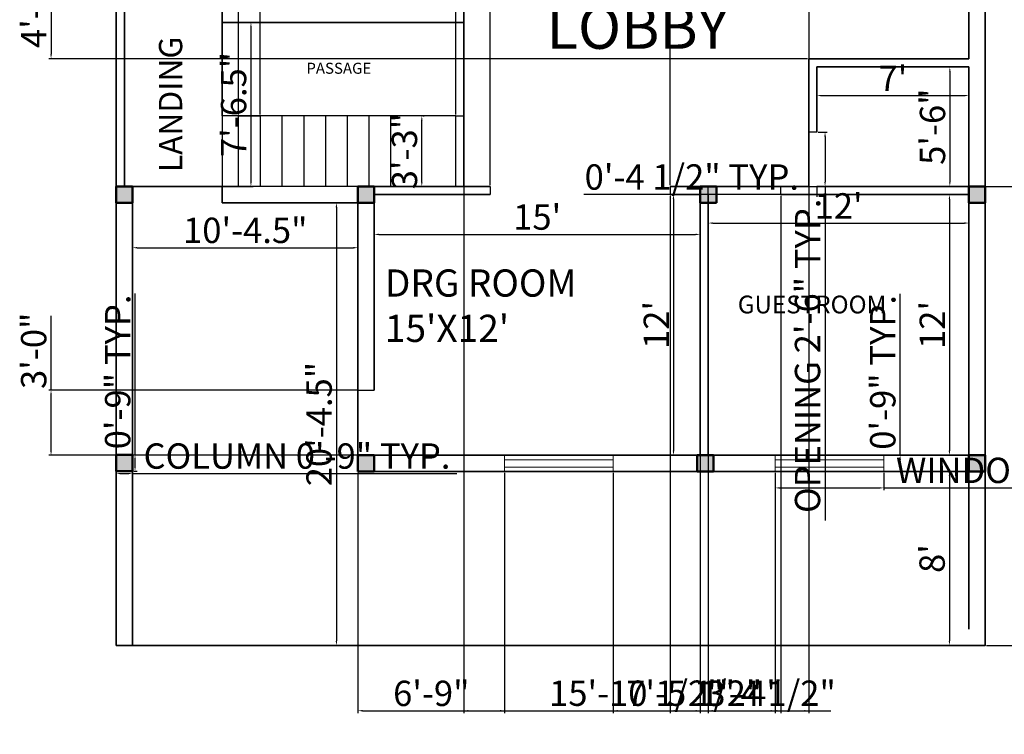
# Model space of a CAD drawing. Units: inches. Extents: x 3316 to 4157, y 2203 to 2977.
# Tile 1 of 4: x 3316 to 3860, y 2203 to 2597. Entities that reach past the tile are written whole.
import ezdxf

# ---------------------------------------------------------------- set-up
doc = ezdxf.new("R2010")
doc.units = ezdxf.units.IN
for name, color, linetype, lineweight in [('A-ANNO-DIMS', 2, 'Continuous', 18), ('A-AREA-IDEN', 7, 'Continuous', 25), ('A-COLS', 7, 'Continuous', 50), ('A-COLS-PATT', 4, 'Continuous', 13), ('A-DOOR', 3, 'Continuous', 25), ('A-FLOR-STRS', 7, 'Continuous', 25), ('A-GLAZ', 4, 'Continuous', 18), ('A-WALL', 7, 'Continuous', 35), ('C-PROP', 7, 'Continuous', 35)]:
    doc.layers.add(name, color=color, linetype=linetype, lineweight=lineweight)
doc.styles.get("Standard").update_dxf_attribs({"font": 'arial.ttf'})
doc.dimstyles.new('ISO-25', dxfattribs={"dimtxt": 14, "dimasz": 2.5, "dimexe": 1.25, "dimexo": 0.625, "dimtad": 1, "dimlunit": 3, "dimtxsty": 'Standard', "dimcen": 2.5, "dimadec": 0, "dimazin": 0, "dimtfac": 1, "dimtmove": 0, "dimatfit": 3, "dimfxl": 1, "dimarcsym": 0})

# ---------------------------------------------------------------- blocks, each defined once
blk = doc.blocks.new('*D4')
at = {"layer": 'A-ANNO-DIMS', "color": 0, "lineweight": -2, "transparency": 16777216}
for p, q in [((3829.8, 2345.34), (3829.8, 2254.34)), ((3830.42, 2347.84), (3831.05, 2347.84)), ((3826.44, 2251.84), (3831.05, 2251.84))]:
    blk.add_line(p, q, dxfattribs=at)
at = {"layer": 'A-ANNO-DIMS', "color": 0, "transparency": 16777216}
for points in [[(3829.38, 2345.34), (3830.21, 2345.34), (3829.8, 2347.84)], [(3829.38, 2254.34), (3830.21, 2254.34), (3829.8, 2251.84)]]:
    blk.add_solid(points, dxfattribs=at)
at = {"layer": 'Defpoints', "color": 0, "transparency": 16777216}
for p in [(3829.8, 2347.84), (3825.82, 2251.84), (3829.8, 2251.84)]:
    blk.add_point(p, dxfattribs=at)
at = {"layer": 'A-ANNO-DIMS', "color": 0, "transparency": 16777216, "insert": (3822.02, 2299.84), "char_height": 14, "attachment_point": 5, "rotation": 90}
blk.add_mtext("8'", dxfattribs=at)
blk = doc.blocks.new('*D5')
at = {"layer": 'A-ANNO-DIMS', "color": 0, "lineweight": -2, "transparency": 16777216}
for p, q in [((3677.36, 2498.34), (3677.36, 2359.34)), ((3677.99, 2500.84), (3678.61, 2500.84)), ((3532.24, 2356.84), (3678.61, 2356.84))]:
    blk.add_line(p, q, dxfattribs=at)
at = {"layer": 'A-ANNO-DIMS', "color": 0, "transparency": 16777216}
for points in [[(3676.94, 2498.34), (3677.78, 2498.34), (3677.36, 2500.84)], [(3676.94, 2359.34), (3677.78, 2359.34), (3677.36, 2356.84)]]:
    blk.add_solid(points, dxfattribs=at)
at = {"layer": 'Defpoints', "color": 0, "transparency": 16777216}
for p in [(3677.36, 2500.84), (3531.62, 2356.84), (3677.36, 2356.84)]:
    blk.add_point(p, dxfattribs=at)
at = {"layer": 'A-ANNO-DIMS', "color": 0, "transparency": 16777216, "insert": (3669.71, 2428.84), "char_height": 14, "attachment_point": 5, "rotation": 90}
blk.add_mtext("12'", dxfattribs=at)
blk = doc.blocks.new('*D7')
at = {"layer": 'A-ANNO-DIMS', "color": 0, "lineweight": -2, "transparency": 16777216}
for p, q in [((3850.21, 2887.84), (4040.36, 2887.84)), ((4039.11, 2885.34), (4039.11, 2254.34)), ((3850.21, 2251.84), (4040.36, 2251.84))]:
    blk.add_line(p, q, dxfattribs=at)
at = {"layer": 'A-ANNO-DIMS', "color": 0, "transparency": 16777216}
for points in [[(4038.69, 2885.34), (4039.53, 2885.34), (4039.11, 2887.84)], [(4038.69, 2254.34), (4039.53, 2254.34), (4039.11, 2251.84)]]:
    blk.add_solid(points, dxfattribs=at)
at = {"layer": 'Defpoints', "color": 0, "transparency": 16777216}
for p in [(3849.58, 2887.84), (3849.58, 2251.84), (4039.11, 2251.84)]:
    blk.add_point(p, dxfattribs=at)
at = {"layer": 'A-ANNO-DIMS', "color": 0, "transparency": 16777216, "insert": (4031.33, 2569.84), "char_height": 14, "attachment_point": 5, "rotation": 90}
blk.add_mtext("53'", dxfattribs=at)
blk = doc.blocks.new('*D12')
at = {"layer": 'A-ANNO-DIMS', "color": 0, "lineweight": -2, "transparency": 16777216}
for p, q in [((3538.33, 2507.84), (3538.33, 2541.84)), ((3538.96, 2544.34), (3539.58, 2544.34)), ((3538.96, 2505.34), (3539.58, 2505.34))]:
    blk.add_line(p, q, dxfattribs=at)
at = {"layer": 'A-ANNO-DIMS', "color": 0, "transparency": 16777216}
for points in [[(3537.91, 2541.84), (3538.75, 2541.84), (3538.33, 2544.34)], [(3537.91, 2507.84), (3538.75, 2507.84), (3538.33, 2505.34)]]:
    blk.add_solid(points, dxfattribs=at)
at = {"layer": 'Defpoints', "color": 0, "transparency": 16777216}
for p in [(3538.33, 2544.34), (3538.33, 2544.34), (3538.33, 2505.34)]:
    blk.add_point(p, dxfattribs=at)
at = {"layer": 'A-ANNO-DIMS', "color": 0, "transparency": 16777216, "insert": (3530.55, 2524.84), "char_height": 14, "attachment_point": 5, "rotation": 90}
blk.add_mtext('3\'-3"', dxfattribs=at)
blk = doc.blocks.new('*D13')
at = {"layer": 'A-ANNO-DIMS', "color": 0, "lineweight": -2, "transparency": 16777216}
for p, q in [((3428.71, 2595.84), (3445.21, 2595.84)), ((3443.96, 2593.34), (3443.96, 2507.84)), ((3428.71, 2505.34), (3445.21, 2505.34))]:
    blk.add_line(p, q, dxfattribs=at)
at = {"layer": 'A-ANNO-DIMS', "color": 0, "transparency": 16777216}
for points in [[(3443.54, 2593.34), (3444.37, 2593.34), (3443.96, 2595.84)], [(3443.54, 2507.84), (3444.37, 2507.84), (3443.96, 2505.34)]]:
    blk.add_solid(points, dxfattribs=at)
at = {"layer": 'Defpoints', "color": 0, "transparency": 16777216}
for p in [(3428.08, 2595.84), (3428.08, 2505.34), (3443.96, 2505.34)]:
    blk.add_point(p, dxfattribs=at)
at = {"layer": 'A-ANNO-DIMS', "color": 0, "transparency": 16777216, "insert": (3436.19, 2550.59), "char_height": 14, "attachment_point": 5, "rotation": 90}
blk.add_mtext('7\'-6.5"', dxfattribs=at)
blk = doc.blocks.new('*D18')
at = {"layer": 'A-ANNO-DIMS', "color": 0, "lineweight": -2, "transparency": 16777216}
for p, q in [((3839.96, 2571.34), (3828.76, 2571.34)), ((3830.01, 2568.84), (3830.01, 2507.84)), ((3839.96, 2505.34), (3828.76, 2505.34))]:
    blk.add_line(p, q, dxfattribs=at)
at = {"layer": 'A-ANNO-DIMS', "color": 0, "transparency": 16777216}
for points in [[(3829.59, 2568.84), (3830.42, 2568.84), (3830.01, 2571.34)], [(3829.59, 2507.84), (3830.42, 2507.84), (3830.01, 2505.34)]]:
    blk.add_solid(points, dxfattribs=at)
at = {"layer": 'Defpoints', "color": 0, "transparency": 16777216}
for p in [(3840.58, 2571.34), (3830.01, 2505.34), (3840.58, 2505.34)]:
    blk.add_point(p, dxfattribs=at)
at = {"layer": 'A-ANNO-DIMS', "color": 0, "transparency": 16777216, "insert": (3822.24, 2538.34), "char_height": 14, "attachment_point": 5, "rotation": 90}
blk.add_mtext('5\'-6"', dxfattribs=at)
blk = doc.blocks.new('*D19')
at = {"layer": 'A-ANNO-DIMS', "color": 0, "lineweight": -2, "transparency": 16777216}
for p, q in [((3756.58, 2570.72), (3756.58, 2554.25)), ((3840.58, 2570.72), (3840.58, 2554.25)), ((3759.08, 2555.5), (3838.08, 2555.5))]:
    blk.add_line(p, q, dxfattribs=at)
at = {"layer": 'A-ANNO-DIMS', "color": 0, "transparency": 16777216}
for points in [[(3759.08, 2555.91), (3759.08, 2555.08), (3756.58, 2555.5)], [(3838.08, 2555.91), (3838.08, 2555.08), (3840.58, 2555.5)]]:
    blk.add_solid(points, dxfattribs=at)
at = {"layer": 'Defpoints', "color": 0, "transparency": 16777216}
for p in [(3756.58, 2571.34), (3840.58, 2571.34), (3840.58, 2555.5)]:
    blk.add_point(p, dxfattribs=at)
at = {"layer": 'A-ANNO-DIMS', "color": 0, "transparency": 16777216, "insert": (3798.58, 2563.12), "char_height": 14, "attachment_point": 5}
blk.add_mtext("7'", dxfattribs=at)
blk = doc.blocks.new('*D20')
at = {"layer": 'A-ANNO-DIMS', "color": 0, "lineweight": -2, "transparency": 16777216}
for p, q in [((3839.96, 2500.84), (3828.55, 2500.84)), ((3829.8, 2498.34), (3829.8, 2359.34)), ((3839.96, 2356.84), (3828.55, 2356.84))]:
    blk.add_line(p, q, dxfattribs=at)
at = {"layer": 'A-ANNO-DIMS', "color": 0, "transparency": 16777216}
for points in [[(3829.38, 2498.34), (3830.21, 2498.34), (3829.8, 2500.84)], [(3829.38, 2359.34), (3830.21, 2359.34), (3829.8, 2356.84)]]:
    blk.add_solid(points, dxfattribs=at)
at = {"layer": 'Defpoints', "color": 0, "transparency": 16777216}
for p in [(3840.58, 2500.84), (3829.8, 2356.84), (3840.58, 2356.84)]:
    blk.add_point(p, dxfattribs=at)
at = {"layer": 'A-ANNO-DIMS', "color": 0, "transparency": 16777216, "insert": (3822.14, 2428.84), "char_height": 14, "attachment_point": 5, "rotation": 90}
blk.add_mtext("12'", dxfattribs=at)
blk = doc.blocks.new('*D21')
at = {"layer": 'A-ANNO-DIMS', "color": 0, "lineweight": -2, "transparency": 16777216}
for p, q in [((3696.58, 2357.47), (3696.58, 2486.34)), ((3840.58, 2357.47), (3840.58, 2486.34)), ((3699.08, 2485.09), (3838.08, 2485.09))]:
    blk.add_line(p, q, dxfattribs=at)
at = {"layer": 'A-ANNO-DIMS', "color": 0, "transparency": 16777216}
for points in [[(3699.08, 2485.51), (3699.08, 2484.68), (3696.58, 2485.09)], [(3838.08, 2485.51), (3838.08, 2484.68), (3840.58, 2485.09)]]:
    blk.add_solid(points, dxfattribs=at)
at = {"layer": 'Defpoints', "color": 0, "transparency": 16777216}
for p in [(3840.58, 2485.09), (3696.58, 2356.84), (3840.58, 2356.84)]:
    blk.add_point(p, dxfattribs=at)
at = {"layer": 'A-ANNO-DIMS', "color": 0, "transparency": 16777216, "insert": (3768.58, 2492.75), "char_height": 14, "attachment_point": 5}
blk.add_mtext("12'", dxfattribs=at)
blk = doc.blocks.new('*D24')
at = {"layer": 'A-ANNO-DIMS', "color": 0, "lineweight": -2, "transparency": 16777216}
for p, q in [((3378.58, 2504.72), (3378.58, 2470.22)), ((3503.08, 2495.72), (3503.08, 2470.22)), ((3381.08, 2471.47), (3500.58, 2471.47))]:
    blk.add_line(p, q, dxfattribs=at)
at = {"layer": 'A-ANNO-DIMS', "color": 0, "transparency": 16777216}
for points in [[(3381.08, 2471.89), (3381.08, 2471.06), (3378.58, 2471.47)], [(3500.58, 2471.89), (3500.58, 2471.06), (3503.08, 2471.47)]]:
    blk.add_solid(points, dxfattribs=at)
at = {"layer": 'Defpoints', "color": 0, "transparency": 16777216}
for p in [(3378.58, 2505.34), (3503.08, 2496.34), (3503.08, 2471.47)]:
    blk.add_point(p, dxfattribs=at)
at = {"layer": 'A-ANNO-DIMS', "color": 0, "transparency": 16777216, "insert": (3440.83, 2479.25), "char_height": 14, "attachment_point": 5}
blk.add_mtext('10\'-4.5"', dxfattribs=at)
blk = doc.blocks.new('*D25')
at = {"layer": 'A-ANNO-DIMS', "color": 0, "lineweight": -2, "transparency": 16777216}
for p, q in [((3502.46, 2496.34), (3489.92, 2496.34)), ((3491.17, 2493.84), (3491.17, 2254.34)), ((3502.46, 2251.84), (3489.92, 2251.84))]:
    blk.add_line(p, q, dxfattribs=at)
at = {"layer": 'A-ANNO-DIMS', "color": 0, "transparency": 16777216}
for points in [[(3490.75, 2493.84), (3491.59, 2493.84), (3491.17, 2496.34)], [(3490.75, 2254.34), (3491.59, 2254.34), (3491.17, 2251.84)]]:
    blk.add_solid(points, dxfattribs=at)
at = {"layer": 'Defpoints', "color": 0, "transparency": 16777216}
for p in [(3503.08, 2496.34), (3491.17, 2251.84), (3503.08, 2251.84)]:
    blk.add_point(p, dxfattribs=at)
at = {"layer": 'A-ANNO-DIMS', "color": 0, "transparency": 16777216, "insert": (3483.4, 2374.09), "char_height": 14, "attachment_point": 5, "rotation": 90}
blk.add_mtext('20\'-4.5"', dxfattribs=at)
blk = doc.blocks.new('*D27')
at = {"layer": 'A-ANNO-DIMS', "color": 0, "lineweight": -2, "transparency": 16777216}
for p, q in [((3512.08, 2500.22), (3512.08, 2477.57)), ((3692.08, 2500.22), (3692.08, 2477.57)), ((3514.58, 2478.82), (3689.58, 2478.82))]:
    blk.add_line(p, q, dxfattribs=at)
at = {"layer": 'A-ANNO-DIMS', "color": 0, "transparency": 16777216}
for points in [[(3514.58, 2479.24), (3514.58, 2478.4), (3512.08, 2478.82)], [(3689.58, 2479.24), (3689.58, 2478.4), (3692.08, 2478.82)]]:
    blk.add_solid(points, dxfattribs=at)
at = {"layer": 'Defpoints', "color": 0, "transparency": 16777216}
for p in [(3512.08, 2500.84), (3692.08, 2500.84), (3692.08, 2478.82)]:
    blk.add_point(p, dxfattribs=at)
at = {"layer": 'A-ANNO-DIMS', "color": 0, "transparency": 16777216, "insert": (3602.08, 2486.59), "char_height": 14, "attachment_point": 5}
blk.add_mtext("15'", dxfattribs=at)
blk = doc.blocks.new('COL-9IN-SQ')
for p, q in [((0, 9), (0, 0)), ((9, 9), (0, 9)), ((9, 0), (9, 9)), ((0, 0), (9, 0))]:
    blk.add_line(p, q)
blk = doc.blocks.new('WIN-60IN')
for p, q in [((0, 0), (0, 9)), ((60, 6.5), (0, 6.5)), ((60, 9), (60, 0)), ((60, 2.5), (0, 2.5)), ((60, 0), (0, 0))]:
    blk.add_line(p, q)
blk = doc.blocks.new('DOOR-30IN-OPENING')
for p, q in [((4.5, 30), (0, 30)), ((4.5, 0), (4.5, 30)), ((0, 0), (4.5, 0))]:
    blk.add_line(p, q)
blk = doc.blocks.new('*D34')
at = {"layer": 'A-ANNO-DIMS', "color": 0, "lineweight": -2, "transparency": 16777216}
for p, q in [((3369.58, 2347.48), (3369.58, 2345.5)), ((3372.08, 2346.75), (3376.08, 2346.75)), ((3378.58, 2347.48), (3378.58, 2345.5)), ((3378.58, 2346.75), (3557.7, 2346.75))]:
    blk.add_line(p, q, dxfattribs=at)
at = {"layer": 'A-ANNO-DIMS', "color": 0, "transparency": 16777216}
for points in [[(3372.08, 2347.17), (3372.08, 2346.34), (3369.58, 2346.75)], [(3376.08, 2347.17), (3376.08, 2346.34), (3378.58, 2346.75)]]:
    blk.add_solid(points, dxfattribs=at)
at = {"layer": 'Defpoints', "color": 0, "transparency": 16777216}
for p in [(3369.58, 2348.1), (3378.58, 2348.1), (3378.58, 2346.75)]:
    blk.add_point(p, dxfattribs=at)
at = {"layer": 'A-ANNO-DIMS', "color": 0, "transparency": 16777216, "insert": (3469.39, 2354.62), "char_height": 14, "attachment_point": 5}
blk.add_mtext('COLUMN 0\'-9" TYP.', dxfattribs=at)
blk = doc.blocks.new('*D35')
at = {"layer": 'A-ANNO-DIMS', "color": 0, "lineweight": -2, "transparency": 16777216}
for p, q in [((3379.93, 2357.1), (3379.93, 2446.19)), ((3379.21, 2357.1), (3381.18, 2357.1)), ((3379.93, 2350.6), (3379.93, 2354.6)), ((3379.21, 2348.1), (3381.18, 2348.1))]:
    blk.add_line(p, q, dxfattribs=at)
at = {"layer": 'A-ANNO-DIMS', "color": 0, "transparency": 16777216}
for points in [[(3379.52, 2354.6), (3380.35, 2354.6), (3379.93, 2357.1)], [(3379.52, 2350.6), (3380.35, 2350.6), (3379.93, 2348.1)]]:
    blk.add_solid(points, dxfattribs=at)
at = {"layer": 'Defpoints', "color": 0, "transparency": 16777216}
for p in [(3378.58, 2357.1), (3379.93, 2357.1), (3378.58, 2348.1)]:
    blk.add_point(p, dxfattribs=at)
at = {"layer": 'A-ANNO-DIMS', "color": 0, "transparency": 16777216, "insert": (3372.16, 2402.9), "char_height": 14, "attachment_point": 5, "rotation": 90}
blk.add_mtext('0\'-9" TYP.', dxfattribs=at)
blk = doc.blocks.new('*D38')
at = {"layer": 'A-ANNO-DIMS', "color": 0, "lineweight": -2, "transparency": 16777216}
for p, q in [((3733.56, 2347.22), (3733.56, 2337.59)), ((3793.56, 2347.22), (3793.56, 2337.59)), ((3736.06, 2338.84), (3791.06, 2338.84)), ((3793.56, 2338.84), (3974.47, 2338.84))]:
    blk.add_line(p, q, dxfattribs=at)
at = {"layer": 'A-ANNO-DIMS', "color": 0, "transparency": 16777216}
for points in [[(3736.06, 2339.26), (3736.06, 2338.43), (3733.56, 2338.84)], [(3791.06, 2339.26), (3791.06, 2338.43), (3793.56, 2338.84)]]:
    blk.add_solid(points, dxfattribs=at)
at = {"layer": 'Defpoints', "color": 0, "transparency": 16777216}
for p in [(3733.56, 2347.84), (3793.56, 2347.84), (3793.56, 2338.84)]:
    blk.add_point(p, dxfattribs=at)
at = {"layer": 'A-ANNO-DIMS', "color": 0, "transparency": 16777216, "insert": (3885.26, 2346.71), "char_height": 14, "attachment_point": 5}
blk.add_mtext('WINDOW 5\'-0" TYP.', dxfattribs=at)
blk = doc.blocks.new('*D39')
at = {"layer": 'A-ANNO-DIMS', "color": 0, "lineweight": -2, "transparency": 16777216}
for p, q in [((3802.56, 2356.84), (3802.56, 2445.93)), ((3794.18, 2356.84), (3803.81, 2356.84)), ((3802.56, 2350.34), (3802.56, 2354.34)), ((3794.18, 2347.84), (3803.81, 2347.84))]:
    blk.add_line(p, q, dxfattribs=at)
at = {"layer": 'A-ANNO-DIMS', "color": 0, "transparency": 16777216}
for points in [[(3802.14, 2354.34), (3802.98, 2354.34), (3802.56, 2356.84)], [(3802.14, 2350.34), (3802.98, 2350.34), (3802.56, 2347.84)]]:
    blk.add_solid(points, dxfattribs=at)
at = {"layer": 'Defpoints', "color": 0, "transparency": 16777216}
for p in [(3793.56, 2356.84), (3802.56, 2356.84), (3793.56, 2347.84)]:
    blk.add_point(p, dxfattribs=at)
at = {"layer": 'A-ANNO-DIMS', "color": 0, "transparency": 16777216, "insert": (3794.79, 2402.64), "char_height": 14, "attachment_point": 5, "rotation": 90}
blk.add_mtext('0\'-9" TYP.', dxfattribs=at)
blk = doc.blocks.new('*D44')
at = {"layer": 'A-ANNO-DIMS', "color": 0, "lineweight": -2, "transparency": 16777216}
for p, q in [((3757.21, 2535.34), (3762.33, 2535.34)), ((3761.08, 2532.84), (3761.08, 2507.84)), ((3757.21, 2505.34), (3762.33, 2505.34)), ((3761.08, 2505.34), (3761.08, 2320.76))]:
    blk.add_line(p, q, dxfattribs=at)
at = {"layer": 'A-ANNO-DIMS', "color": 0, "transparency": 16777216}
for points in [[(3760.67, 2532.84), (3761.5, 2532.84), (3761.08, 2535.34)], [(3760.67, 2507.84), (3761.5, 2507.84), (3761.08, 2505.34)]]:
    blk.add_solid(points, dxfattribs=at)
at = {"layer": 'Defpoints', "color": 0, "transparency": 16777216}
for p in [(3756.58, 2535.34), (3756.58, 2505.34), (3761.08, 2505.34)]:
    blk.add_point(p, dxfattribs=at)
at = {"layer": 'A-ANNO-DIMS', "color": 0, "transparency": 16777216, "insert": (3753.22, 2411.8), "char_height": 14, "attachment_point": 5, "rotation": 90}
blk.add_mtext('OPENING 2\'-6" TYP.', dxfattribs=at)
blk = doc.blocks.new('*D45')
at = {"layer": 'A-ANNO-DIMS', "color": 0, "lineweight": -2, "transparency": 16777216}
for p, q in [((3752.08, 2504.72), (3752.08, 2499.59)), ((3756.58, 2504.72), (3756.58, 2499.59)), ((3749.58, 2500.84), (3627.87, 2500.84)), ((3756.58, 2500.84), (3752.08, 2500.84)), ((3759.08, 2500.84), (3761.58, 2500.84))]:
    blk.add_line(p, q, dxfattribs=at)
at = {"layer": 'A-ANNO-DIMS', "color": 0, "transparency": 16777216}
for points in [[(3749.58, 2501.26), (3749.58, 2500.43), (3752.08, 2500.84)], [(3759.08, 2501.26), (3759.08, 2500.43), (3756.58, 2500.84)]]:
    blk.add_solid(points, dxfattribs=at)
at = {"layer": 'Defpoints', "color": 0, "transparency": 16777216}
for p in [(3752.08, 2505.34), (3756.58, 2505.34), (3752.08, 2500.84)]:
    blk.add_point(p, dxfattribs=at)
at = {"layer": 'A-ANNO-DIMS', "color": 0, "transparency": 16777216, "insert": (3687.48, 2508.71), "char_height": 14, "attachment_point": 5}
blk.add_mtext('0\'-4 1/2" TYP.', dxfattribs=at)
blk = doc.blocks.new('*D46')
at = {"layer": 'A-ANNO-DIMS', "color": 0, "lineweight": -2, "transparency": 16777216}
for p, q in [((3503.08, 2347.22), (3503.08, 2214.54)), ((3584.09, 2347.22), (3584.09, 2214.54)), ((3505.58, 2215.79), (3581.59, 2215.79))]:
    blk.add_line(p, q, dxfattribs=at)
at = {"layer": 'A-ANNO-DIMS', "color": 0, "transparency": 16777216}
for points in [[(3505.58, 2216.21), (3505.58, 2215.38), (3503.08, 2215.79)], [(3581.59, 2216.21), (3581.59, 2215.38), (3584.09, 2215.79)]]:
    blk.add_solid(points, dxfattribs=at)
at = {"layer": 'Defpoints', "color": 0, "transparency": 16777216}
for p in [(3503.08, 2347.84), (3584.09, 2347.84), (3584.09, 2215.79)]:
    blk.add_point(p, dxfattribs=at)
at = {"layer": 'A-ANNO-DIMS', "color": 0, "transparency": 16777216, "insert": (3543.59, 2223.57), "char_height": 14, "attachment_point": 5}
blk.add_mtext('6\'-9"', dxfattribs=at)
blk = doc.blocks.new('*D47')
at = {"layer": 'A-ANNO-DIMS', "color": 0, "lineweight": -2, "transparency": 16777216}
for p, q in [((3644.09, 2347.22), (3644.09, 2214.54)), ((3733.56, 2347.22), (3733.56, 2214.54)), ((3646.59, 2215.79), (3731.06, 2215.79))]:
    blk.add_line(p, q, dxfattribs=at)
at = {"layer": 'A-ANNO-DIMS', "color": 0, "transparency": 16777216}
for points in [[(3646.59, 2216.21), (3646.59, 2215.38), (3644.09, 2215.79)], [(3731.06, 2216.21), (3731.06, 2215.38), (3733.56, 2215.79)]]:
    blk.add_solid(points, dxfattribs=at)
at = {"layer": 'Defpoints', "color": 0, "transparency": 16777216}
for p in [(3644.09, 2347.84), (3733.56, 2347.84), (3733.56, 2215.79)]:
    blk.add_point(p, dxfattribs=at)
at = {"layer": 'A-ANNO-DIMS', "color": 0, "transparency": 16777216, "insert": (3688.82, 2223.66), "char_height": 14, "attachment_point": 5}
blk.add_mtext('7\'-5 1/2"', dxfattribs=at)
blk = doc.blocks.new('*D50')
at = {"layer": 'A-ANNO-DIMS', "color": 0, "lineweight": -2, "transparency": 16777216}
for p, q in [((3751.46, 2629.84), (3332.28, 2629.84)), ((3333.53, 2627.34), (3333.53, 2578.34)), ((3751.46, 2575.84), (3332.28, 2575.84))]:
    blk.add_line(p, q, dxfattribs=at)
at = {"layer": 'A-ANNO-DIMS', "color": 0, "transparency": 16777216}
for points in [[(3333.12, 2627.34), (3333.95, 2627.34), (3333.53, 2629.84)], [(3333.12, 2578.34), (3333.95, 2578.34), (3333.53, 2575.84)]]:
    blk.add_solid(points, dxfattribs=at)
at = {"layer": 'Defpoints', "color": 0, "transparency": 16777216}
for p in [(3752.08, 2629.84), (3333.53, 2575.84), (3752.08, 2575.84)]:
    blk.add_point(p, dxfattribs=at)
at = {"layer": 'A-ANNO-DIMS', "color": 0, "transparency": 16777216, "insert": (3325.76, 2602.84), "char_height": 14, "attachment_point": 5, "rotation": 90}
blk.add_mtext('4\'-6"', dxfattribs=at)
blk = doc.blocks.new('*D52')
at = {"layer": 'A-ANNO-DIMS', "color": 0, "lineweight": -2, "transparency": 16777216}
for p, q in [((3576.12, 2505.97), (3576.12, 2925.14)), ((3578.62, 2923.89), (3673.07, 2923.89)), ((3675.57, 2505.97), (3675.57, 2925.14))]:
    blk.add_line(p, q, dxfattribs=at)
at = {"layer": 'A-ANNO-DIMS', "color": 0, "transparency": 16777216}
for points in [[(3578.62, 2924.31), (3578.62, 2923.48), (3576.12, 2923.89)], [(3673.07, 2924.31), (3673.07, 2923.48), (3675.57, 2923.89)]]:
    blk.add_solid(points, dxfattribs=at)
at = {"layer": 'Defpoints', "color": 0, "transparency": 16777216}
for p in [(3675.57, 2923.89), (3576.12, 2505.34), (3675.57, 2505.34)]:
    blk.add_point(p, dxfattribs=at)
at = {"layer": 'A-ANNO-DIMS', "color": 0, "transparency": 16777216, "insert": (3625.84, 2931.76), "char_height": 14, "attachment_point": 5}
blk.add_mtext('8\'-3 1/2"', dxfattribs=at)
blk = doc.blocks.new('*D53')
at = {"layer": 'A-ANNO-DIMS', "color": 0, "lineweight": -2, "transparency": 16777216}
for p, q in [((3675.57, 2500.22), (3675.57, 2214.54)), ((3692.08, 2500.22), (3692.08, 2214.54)), ((3678.07, 2215.79), (3689.58, 2215.79)), ((3692.08, 2215.79), (3764.35, 2215.79))]:
    blk.add_line(p, q, dxfattribs=at)
at = {"layer": 'A-ANNO-DIMS', "color": 0, "transparency": 16777216}
for points in [[(3678.07, 2216.21), (3678.07, 2215.38), (3675.57, 2215.79)], [(3689.58, 2216.21), (3689.58, 2215.38), (3692.08, 2215.79)]]:
    blk.add_solid(points, dxfattribs=at)
at = {"layer": 'Defpoints', "color": 0, "transparency": 16777216}
for p in [(3675.57, 2500.84), (3692.08, 2500.84), (3692.08, 2215.79)]:
    blk.add_point(p, dxfattribs=at)
at = {"layer": 'A-ANNO-DIMS', "color": 0, "transparency": 16777216, "insert": (3729.47, 2223.66), "char_height": 14, "attachment_point": 5}
blk.add_mtext('1\'-4 1/2"', dxfattribs=at)
blk = doc.blocks.new('*D54')
at = {"layer": 'A-ANNO-DIMS', "color": 0, "lineweight": -2, "transparency": 16777216}
for p, q in [((3696.58, 2500.22), (3696.58, 2214.54)), ((3736.58, 2500.22), (3736.58, 2214.54)), ((3699.08, 2215.79), (3734.08, 2215.79))]:
    blk.add_line(p, q, dxfattribs=at)
at = {"layer": 'A-ANNO-DIMS', "color": 0, "transparency": 16777216}
for points in [[(3699.08, 2216.21), (3699.08, 2215.38), (3696.58, 2215.79)], [(3734.08, 2216.21), (3734.08, 2215.38), (3736.58, 2215.79)]]:
    blk.add_solid(points, dxfattribs=at)
at = {"layer": 'Defpoints', "color": 0, "transparency": 16777216}
for p in [(3696.58, 2500.84), (3736.58, 2500.84), (3736.58, 2215.79)]:
    blk.add_point(p, dxfattribs=at)
at = {"layer": 'A-ANNO-DIMS', "color": 0, "transparency": 16777216, "insert": (3716.58, 2223.57), "char_height": 14, "attachment_point": 5}
blk.add_mtext('3\'-4"', dxfattribs=at)
blk = doc.blocks.new('*D55')
at = {"layer": 'A-ANNO-DIMS', "color": 0, "lineweight": -2, "transparency": 16777216}
for p, q in [((3333.53, 2392.84), (3333.53, 2433.8)), ((3502.46, 2392.84), (3332.28, 2392.84)), ((3333.53, 2359.34), (3333.53, 2390.34)), ((3502.46, 2356.84), (3332.28, 2356.84))]:
    blk.add_line(p, q, dxfattribs=at)
at = {"layer": 'A-ANNO-DIMS', "color": 0, "transparency": 16777216}
for points in [[(3333.12, 2390.34), (3333.95, 2390.34), (3333.53, 2392.84)], [(3333.12, 2359.34), (3333.95, 2359.34), (3333.53, 2356.84)]]:
    blk.add_solid(points, dxfattribs=at)
at = {"layer": 'Defpoints', "color": 0, "transparency": 16777216}
for p in [(3333.53, 2392.84), (3503.08, 2392.84), (3503.08, 2356.84)]:
    blk.add_point(p, dxfattribs=at)
at = {"layer": 'A-ANNO-DIMS', "color": 0, "transparency": 16777216, "insert": (3325.76, 2414.57), "char_height": 14, "attachment_point": 5, "rotation": 90}
blk.add_mtext('3\'-0"', dxfattribs=at)
blk = doc.blocks.new('*D56')
at = {"layer": 'A-ANNO-DIMS', "color": 0, "lineweight": -2, "transparency": 16777216}
for p, q in [((3752.08, 2699.72), (3752.08, 2214.54)), ((3561.58, 2662.22), (3561.58, 2214.54)), ((3564.08, 2215.79), (3749.58, 2215.79))]:
    blk.add_line(p, q, dxfattribs=at)
at = {"layer": 'A-ANNO-DIMS', "color": 0, "transparency": 16777216}
for points in [[(3564.08, 2216.21), (3564.08, 2215.38), (3561.58, 2215.79)], [(3749.58, 2216.21), (3749.58, 2215.38), (3752.08, 2215.79)]]:
    blk.add_solid(points, dxfattribs=at)
at = {"layer": 'Defpoints', "color": 0, "transparency": 16777216}
for p in [(3752.08, 2700.34), (3561.58, 2662.84), (3752.08, 2215.79)]:
    blk.add_point(p, dxfattribs=at)
at = {"layer": 'A-ANNO-DIMS', "color": 0, "transparency": 16777216, "insert": (3656.83, 2223.66), "char_height": 14, "attachment_point": 5}
blk.add_mtext('15\'-10 1/2"', dxfattribs=at)
blk = doc.blocks.new('*D57')
at = {"layer": 'A-ANNO-DIMS', "color": 0, "lineweight": -2, "transparency": 16777216}
for p, q in [((3692.71, 2740.84), (3886.88, 2740.84)), ((3885.63, 2507.84), (3885.63, 2738.34)), ((3676.19, 2505.34), (3886.88, 2505.34))]:
    blk.add_line(p, q, dxfattribs=at)
at = {"layer": 'A-ANNO-DIMS', "color": 0, "transparency": 16777216}
for points in [[(3885.22, 2738.34), (3886.05, 2738.34), (3885.63, 2740.84)], [(3885.22, 2507.84), (3886.05, 2507.84), (3885.63, 2505.34)]]:
    blk.add_solid(points, dxfattribs=at)
at = {"layer": 'Defpoints', "color": 0, "transparency": 16777216}
for p in [(3692.08, 2740.84), (3885.63, 2740.84), (3675.57, 2505.34)]:
    blk.add_point(p, dxfattribs=at)
at = {"layer": 'A-ANNO-DIMS', "color": 0, "transparency": 16777216, "insert": (3877.77, 2623.09), "char_height": 14, "attachment_point": 5, "rotation": 90}
blk.add_mtext('19\'-7 1/2"', dxfattribs=at)
blk = doc.blocks.new('*D59')
at = {"layer": 'A-ANNO-DIMS', "color": 0, "lineweight": -2, "transparency": 16777216}
for p, q in [((3437.08, 2544.97), (3437.08, 2925.14)), ((3439.58, 2923.89), (3446.58, 2923.89)), ((3449.08, 2544.97), (3449.08, 2925.14)), ((3449.08, 2923.89), (3488.73, 2923.89))]:
    blk.add_line(p, q, dxfattribs=at)
at = {"layer": 'A-ANNO-DIMS', "color": 0, "transparency": 16777216}
for points in [[(3439.58, 2924.31), (3439.58, 2923.48), (3437.08, 2923.89)], [(3446.58, 2924.31), (3446.58, 2923.48), (3449.08, 2923.89)]]:
    blk.add_solid(points, dxfattribs=at)
at = {"layer": 'Defpoints', "color": 0, "transparency": 16777216}
for p in [(3449.08, 2923.89), (3437.08, 2544.34), (3449.08, 2544.34)]:
    blk.add_point(p, dxfattribs=at)
at = {"layer": 'A-ANNO-DIMS', "color": 0, "transparency": 16777216, "insert": (3470.16, 2931.67), "char_height": 14, "attachment_point": 5}
blk.add_mtext('1\'-0"', dxfattribs=at)
blk = doc.blocks.new('*D60')
at = {"layer": 'A-ANNO-DIMS', "color": 0, "lineweight": -2, "transparency": 16777216}
for p, q in [((3428.08, 2544.97), (3428.08, 2925.14)), ((3430.58, 2923.89), (3554.58, 2923.89)), ((3557.08, 2544.97), (3557.08, 2925.14))]:
    blk.add_line(p, q, dxfattribs=at)
at = {"layer": 'A-ANNO-DIMS', "color": 0, "transparency": 16777216}
for points in [[(3430.58, 2924.31), (3430.58, 2923.48), (3428.08, 2923.89)], [(3554.58, 2924.31), (3554.58, 2923.48), (3557.08, 2923.89)]]:
    blk.add_solid(points, dxfattribs=at)
at = {"layer": 'Defpoints', "color": 0, "transparency": 16777216}
for p in [(3557.08, 2923.89), (3428.08, 2544.34), (3557.08, 2544.34)]:
    blk.add_point(p, dxfattribs=at)
at = {"layer": 'A-ANNO-DIMS', "color": 0, "transparency": 16777216, "insert": (3492.58, 2931.67), "char_height": 14, "attachment_point": 5}
blk.add_mtext('10\'-9"', dxfattribs=at)

msp = doc.modelspace()

# ---------------------------------------------------------------- hatches: boundary and pattern name
at = {"layer": 'A-COLS-PATT'}
h = msp.add_hatch(color=256, dxfattribs=at)
h.dxf.hatch_style = 1
h.paths.add_polyline_path([(3849.584, 2887.842), (3840.584, 2887.842), (3840.584, 2878.842), (3849.584, 2878.842)])
h.paths.add_polyline_path([(3696.584, 2887.842), (3687.584, 2887.842), (3687.584, 2878.842), (3696.584, 2878.842)])
h.paths.add_polyline_path([(3527.084, 2887.842), (3518.084, 2887.842), (3518.084, 2878.842), (3527.084, 2878.842)])
h.paths.add_polyline_path([(3378.584, 2887.842), (3369.584, 2887.842), (3369.584, 2878.842), (3378.584, 2878.842)])
h.paths.add_polyline_path([(3378.584, 2707.842), (3369.584, 2707.842), (3369.584, 2698.842), (3378.584, 2698.842)])
h.paths.add_polyline_path([(3561.584, 2704.842), (3552.584, 2704.842), (3552.584, 2695.842), (3561.584, 2695.842)])
h.paths.add_polyline_path([(3701.03, 2704.842), (3692.084, 2704.842), (3692.084, 2700.342), (3701.03, 2700.342)])
h.paths.add_polyline_path([(3701.03, 2700.342), (3692.03, 2700.342), (3692.03, 2695.842), (3701.03, 2695.842)])
h.paths.add_polyline_path([(3849.584, 2704.835), (3840.584, 2704.835), (3840.584, 2695.835), (3849.584, 2695.835)])
h.paths.add_polyline_path([(3378.584, 2505.342), (3369.584, 2505.342), (3369.584, 2496.342), (3378.584, 2496.342)])
h.paths.add_polyline_path([(3378.584, 2357.104), (3369.584, 2357.104), (3369.584, 2348.104), (3378.584, 2348.104)])
h.paths.add_polyline_path([(3512.084, 2505.342), (3503.084, 2505.342), (3503.084, 2496.342), (3512.084, 2496.342)])
h.paths.add_polyline_path([(3512.084, 2356.842), (3503.084, 2356.842), (3503.084, 2347.842), (3512.084, 2347.842)])
h.paths.add_polyline_path([(3701.115, 2505.342), (3696.584, 2505.342), (3696.584, 2500.842), (3696.584, 2496.342), (3701.115, 2496.342)])
h.paths.add_polyline_path([(3696.584, 2505.342), (3692.115, 2505.342), (3692.115, 2496.342), (3696.584, 2496.342), (3696.584, 2500.842)])
h.paths.add_polyline_path([(3699.422, 2356.842), (3690.422, 2356.842), (3690.422, 2347.842), (3699.422, 2347.842)])
h.paths.add_polyline_path([(3849.584, 2356.899), (3840.584, 2356.899), (3840.584, 2347.899), (3849.584, 2347.899)])
h.paths.add_polyline_path([(3849.584, 2505.307), (3840.584, 2505.307), (3840.584, 2496.307), (3849.584, 2496.307)])

# ---------------------------------------------------------------- linework, layer by layer
at = {"layer": 'A-DOOR'}
for p, q in [((3576.116, 2505.342), (3576.116, 2500.842)), ((3675.569, 2505.342), (3675.569, 2500.842)), ((3696.584, 2500.842), (3696.584, 2505.342)), ((3736.584, 2500.842), (3736.584, 2505.342)), ((3503.084, 2356.842), (3503.084, 2392.842)), ((3503.084, 2392.842), (3512.084, 2392.842)), ((3512.084, 2356.842), (3503.084, 2356.842))]:
    msp.add_line(p, q, dxfattribs=at)
at = {"layer": 'A-FLOR-STRS'}
for p, q in [((3437.084, 2544.342), (3428.084, 2544.342)), ((3428.084, 2544.342), (3428.084, 2505.342)), ((3557.084, 2544.342), (3428.084, 2544.342)), ((3437.084, 2505.342), (3437.084, 2544.342)), ((3437.084, 2544.342), (3449.084, 2544.342)), ((3449.084, 2544.342), (3449.084, 2505.342)), ((3461.084, 2544.342), (3461.084, 2505.342)), ((3473.084, 2544.342), (3473.084, 2505.342)), ((3485.084, 2544.342), (3485.084, 2505.342)), ((3497.084, 2544.342), (3497.084, 2505.342)), ((3509.084, 2544.342), (3509.084, 2505.342)), ((3521.084, 2544.342), (3521.084, 2505.342)), ((3557.084, 2505.342), (3557.084, 2544.342)), ((3557.084, 2544.342), (3561.584, 2544.342)), ((3557.084, 2505.342), (3437.084, 2505.342))]:
    msp.add_line(p, q, dxfattribs=at)
at = {"layer": 'A-WALL'}
for p, q in [((3374.084, 2505.342), (3374.084, 2698.842)), ((3561.584, 2595.842), (3561.584, 2662.842)), ((3840.584, 2629.842), (3840.584, 2575.842)), ((3428.084, 2601.842), (3428.084, 2595.842)), ((3428.084, 2595.842), (3437.084, 2595.842)), ((3428.084, 2595.842), (3428.084, 2544.342)), ((3437.084, 2595.842), (3557.084, 2595.842)), ((3557.084, 2595.842), (3561.584, 2595.842)), ((3561.584, 2595.842), (3561.584, 2508.842)), ((3561.584, 2595.842), (3561.584, 2547.842)), ((3840.584, 2575.842), (3752.084, 2575.842)), ((3752.084, 2505.342), (3752.084, 2575.842)), ((3840.584, 2571.342), (3756.584, 2571.342)), ((3756.584, 2571.342), (3756.584, 2535.342)), ((3840.584, 2571.342), (3840.584, 2505.342)), ((3561.584, 2508.842), (3561.584, 2505.342)), ((3378.584, 2505.342), (3374.084, 2505.342)), ((3437.084, 2505.342), (3378.584, 2505.342)), ((3378.584, 2251.842), (3378.584, 2505.342)), ((3428.084, 2505.342), (3428.084, 2496.342)), ((3576.116, 2505.342), (3503.084, 2505.342)), ((3561.584, 2505.342), (3557.084, 2505.342)), ((3752.084, 2505.342), (3675.569, 2505.342)), ((3756.584, 2505.342), (3840.584, 2505.342)), ((3512.084, 2500.842), (3512.084, 2392.842)), ((3576.116, 2500.842), (3512.084, 2500.842)), ((3692.084, 2500.842), (3675.569, 2500.842)), ((3692.084, 2356.842), (3692.084, 2500.842)), ((3696.584, 2356.842), (3696.584, 2500.842)), ((3736.584, 2500.842), (3840.584, 2500.842)), ((3840.584, 2500.842), (3752.084, 2500.842)), ((3840.584, 2500.842), (3840.584, 2356.842)), ((3428.084, 2496.342), (3503.084, 2496.342)), ((3503.084, 2356.842), (3503.084, 2496.342)), ((3503.084, 2356.842), (3503.084, 2347.842)), ((3692.084, 2356.842), (3512.084, 2356.842)), ((3840.584, 2356.842), (3696.584, 2356.842)), ((3840.584, 2347.842), (3503.084, 2347.842)), ((3369.584, 2251.842), (3378.584, 2251.842))]:
    msp.add_line(p, q, dxfattribs=at)
for points in [[(3840.584, 2575.842), (3840.584, 2629.842)], [(3840.584, 2505.342), (3840.584, 2571.342)], [(3840.584, 2356.842), (3840.584, 2500.842)], [(3840.584, 2260.842), (3840.584, 2347.842)]]:
    msp.add_lwpolyline(points, dxfattribs=at)
at = {"layer": 'C-PROP'}
msp.add_lwpolyline([(3369.584, 2251.842), (3849.584, 2251.842), (3849.584, 2887.842), (3369.584, 2887.842)], close=True, dxfattribs=at)

# ---------------------------------------------------------------- block references
at = {"layer": 'A-COLS'}
for p in [(3369.584, 2496.342), (3503.084, 2496.342), (3692.115, 2496.342), (3840.584, 2496.308), (3369.584, 2348.104), (3503.084, 2347.842), (3690.422, 2347.842), (3840.584, 2347.899)]:
    msp.add_blockref('COL-9IN-SQ', p, dxfattribs=at)
at = {"layer": 'A-DOOR', "rotation": 180}
msp.add_blockref('DOOR-30IN-OPENING', (3756.583, 2535.342), dxfattribs=at)
at = {"layer": 'A-GLAZ'}
for p in [(3584.087, 2347.842), (3733.558, 2347.842)]:
    msp.add_blockref('WIN-60IN', p, dxfattribs=at)

# ---------------------------------------------------------------- texts
at = {"layer": 'A-AREA-IDEN', "attachment_point": 1}
for s, insert, char_height in [('LOBBY', (3607.117, 2604.899), 23.5794), ('PASSAGE', (3474.56, 2573.622), 6.0899), ('GUESTROOM', (3712.856, 2445.026), 9.8209)]:
    msp.add_mtext(s, dxfattribs=dict(at, insert=insert, char_height=char_height))
at = {"layer": 'A-AREA-IDEN', "insert": (3393.151, 2513.249), "char_height": 12.8375, "attachment_point": 1, "rotation": 90}
msp.add_mtext('LANDING', dxfattribs=at)
at = {"layer": 'A-AREA-IDEN', "insert": (3517.948, 2459.493), "char_height": 15.0175, "attachment_point": 1}
msp.add_mtext_dynamic_manual_height_columns("DRG ROOM\\P15'X12'", width=140.30306, gutter_width=75.087, heights=[0], dxfattribs=at)

# ---------------------------------------------------------------- dimensions: what is measured, and where the dimension line sits
at = {"layer": 'A-ANNO-DIMS'}
for base, p1, p2, override, picture, middle in [((3675.569, 2923.892), (3576.116, 2505.342), (3675.569, 2505.342), {"dimdec": 1, "dimlfac": 1, "dimrnd": 0, "dimzin": 1, "dimdsep": 46, "dimlunit": 4, "dimfrac": 2}, '*D52', (3625.843, 2931.761)), ((3557.084, 2923.892), (3428.084, 2544.342), (3557.084, 2544.342), {"dimdec": 1, "dimlfac": 1, "dimrnd": 0, "dimzin": 1, "dimdsep": 46, "dimlunit": 4, "dimfrac": 2}, '*D60', (3492.584, 2931.665)), ((3449.084, 2923.892), (3437.084, 2544.342), (3449.084, 2544.342), {"dimdec": 1, "dimlfac": 1, "dimrnd": 0, "dimzin": 1, "dimdsep": 46, "dimlunit": 4, "dimfrac": 2}, '*D59', (3470.158, 2931.665)), ((3752.084, 2215.792), (3561.584, 2662.842), (3752.084, 2700.342), {"dimdec": 1, "dimlfac": 1, "dimrnd": 0, "dimzin": 1, "dimdsep": 46, "dimlunit": 4, "dimfrac": 2}, '*D56', (3656.834, 2223.656)), ((3840.584, 2555.498), (3756.584, 2571.342), (3840.584, 2571.342), {"dimclrd": 0, "dimclre": 0, "dimclrt": 0}, '*D19', (3798.584, 2563.123)), ((3503.084, 2471.473), (3378.584, 2505.342), (3503.084, 2496.342), {"dimclrd": 0, "dimclre": 0, "dimclrt": 0}, '*D24', (3440.834, 2479.246)), ((3840.584, 2485.093), (3696.584, 2356.842), (3840.584, 2356.842), {"dimclrd": 0, "dimclre": 0, "dimclrt": 0}, '*D21', (3768.584, 2492.746)), ((3692.084, 2478.819), (3512.084, 2500.842), (3692.084, 2500.842), {"dimclrd": 0, "dimclre": 0, "dimclrt": 0}, '*D27', (3602.084, 2486.592)), ((3692.084, 2215.792), (3675.569, 2500.842), (3692.084, 2500.842), {"dimdec": 1, "dimlfac": 1, "dimrnd": 0, "dimzin": 1, "dimdsep": 46, "dimlunit": 4, "dimfrac": 2}, '*D53', (3729.469, 2223.656)), ((3736.584, 2215.792), (3696.584, 2500.842), (3736.584, 2500.842), {"dimdec": 1, "dimlfac": 1, "dimrnd": 0, "dimzin": 1, "dimdsep": 46, "dimlunit": 4, "dimfrac": 2}, '*D54', (3716.584, 2223.57)), ((3584.087, 2215.792), (3503.084, 2347.842), (3584.087, 2347.842), {"dimdec": 1, "dimlfac": 1, "dimrnd": 0, "dimzin": 1, "dimdsep": 46, "dimlunit": 4, "dimfrac": 2}, '*D46', (3543.585, 2223.565)), ((3733.559, 2215.792), (3644.087, 2347.842), (3733.559, 2347.842), {"dimdec": 1, "dimlfac": 1, "dimrnd": 0, "dimzin": 1, "dimdsep": 46, "dimlunit": 4, "dimfrac": 2}, '*D47', (3688.823, 2223.656))]:
    dim = msp.add_linear_dim(base=base, p1=p1, p2=p2, dimstyle='ISO-25', override=override, dxfattribs=at)
    dim.commit()
    dim.dimension.update_dxf_attribs({"geometry": picture, "text_midpoint": middle})
for base, p1, p2, angle, override, picture, middle in [((4039.111, 2251.842), (3849.584, 2887.842), (3849.584, 2251.842), 90, {"dimclrd": 0, "dimclre": 0, "dimclrt": 0}, '*D7', (4031.333, 2569.842)), ((3885.634, 2740.842), (3675.569, 2505.342), (3692.084, 2740.842), 90, {"dimdec": 1, "dimlfac": 1, "dimrnd": 0, "dimzin": 1, "dimdsep": 46, "dimlunit": 4, "dimfrac": 2}, '*D57', (3877.77, 2623.092)), ((3333.534, 2575.842), (3752.084, 2629.842), (3752.084, 2575.842), 90, {"dimdec": 1, "dimlfac": 1, "dimrnd": 0, "dimzin": 1, "dimdsep": 46, "dimlunit": 4, "dimfrac": 2}, '*D50', (3325.761, 2602.842)), ((3443.958, 2505.342), (3428.084, 2595.842), (3428.084, 2505.342), 90, {"dimclrd": 0, "dimclre": 0, "dimclrt": 0}, '*D13', (3436.185, 2550.592)), ((3830.008, 2505.342), (3840.584, 2571.342), (3840.584, 2505.342), 90, {"dimclrd": 0, "dimclre": 0, "dimclrt": 0}, '*D18', (3822.235, 2538.342)), ((3538.33, 2544.342), (3538.33, 2505.342), (3538.33, 2544.342), 270, {"dimclrd": 0, "dimclre": 0, "dimclrt": 0}, '*D12', (3530.553, 2524.842)), ((3677.361, 2356.842), (3677.361, 2500.842), (3531.618, 2356.842), 270, {"dimclrd": 0, "dimclre": 0, "dimclrt": 0}, '*D5', (3669.708, 2428.842)), ((3829.795, 2356.842), (3840.584, 2500.842), (3840.584, 2356.842), 90, {"dimclrd": 0, "dimclre": 0, "dimclrt": 0}, '*D20', (3822.142, 2428.842)), ((3491.169, 2251.842), (3503.084, 2496.342), (3503.084, 2251.842), 90, {"dimclrd": 0, "dimclre": 0, "dimclrt": 0}, '*D25', (3483.396, 2374.092)), ((3333.534, 2392.842), (3503.084, 2356.842), (3503.084, 2392.842), 90, {"dimdec": 1, "dimlfac": 1, "dimrnd": 0, "dimzin": 1, "dimdsep": 46, "dimlunit": 4, "dimfrac": 2}, '*D55', (3325.756, 2414.57)), ((3829.795, 2251.842), (3829.795, 2347.842), (3825.816, 2251.842), 270, {"dimclrd": 0, "dimclre": 0, "dimclrt": 0}, '*D4', (3822.022, 2299.842))]:
    dim = msp.add_linear_dim(base=base, p1=p1, p2=p2, angle=angle, dimstyle='ISO-25', override=override, dxfattribs=at)
    dim.commit()
    dim.dimension.update_dxf_attribs({"geometry": picture, "text_midpoint": middle})
for base, p1, p2, angle, text, picture, middle in [((3752.084, 2500.842), (3756.584, 2505.342), (3752.084, 2505.342), 180, '<> TYP.', '*D45', (3687.479, 2508.706)), ((3761.084, 2505.342), (3756.584, 2535.342), (3756.584, 2505.342), 270, 'OPENING <> TYP.', '*D44', (3753.215, 2411.8)), ((3379.934, 2357.104), (3378.584, 2348.104), (3378.584, 2357.104), 90, '<> TYP.', '*D35', (3372.161, 2402.897)), ((3802.559, 2356.842), (3793.559, 2347.842), (3793.559, 2356.842), 90, '<> TYP.', '*D39', (3794.785, 2402.636))]:
    dim = msp.add_linear_dim(base=base, p1=p1, p2=p2, angle=angle, text=text, dimstyle='ISO-25', override={"dimdec": 1, "dimlfac": 1, "dimrnd": 0, "dimzin": 1, "dimdsep": 46, "dimlunit": 4, "dimfrac": 2}, dxfattribs=at)
    dim.commit()
    dim.dimension.update_dxf_attribs({"geometry": picture, "text_midpoint": middle})
for base, p1, p2, text, picture, middle in [((3378.584, 2346.754), (3369.584, 2348.104), (3378.584, 2348.104), 'COLUMN <> TYP.', '*D34', (3469.39, 2354.622)), ((3793.559, 2338.842), (3733.559, 2347.842), (3793.559, 2347.842), 'WINDOW <> TYP.', '*D38', (3885.263, 2346.711))]:
    dim = msp.add_linear_dim(base=base, p1=p1, p2=p2, text=text, dimstyle='ISO-25', override={"dimdec": 1, "dimlfac": 1, "dimrnd": 0, "dimzin": 1, "dimdsep": 46, "dimlunit": 4, "dimfrac": 2}, dxfattribs=at)
    dim.commit()
    dim.dimension.update_dxf_attribs({"geometry": picture, "text_midpoint": middle})

doc.saveas('drawing.dxf')
